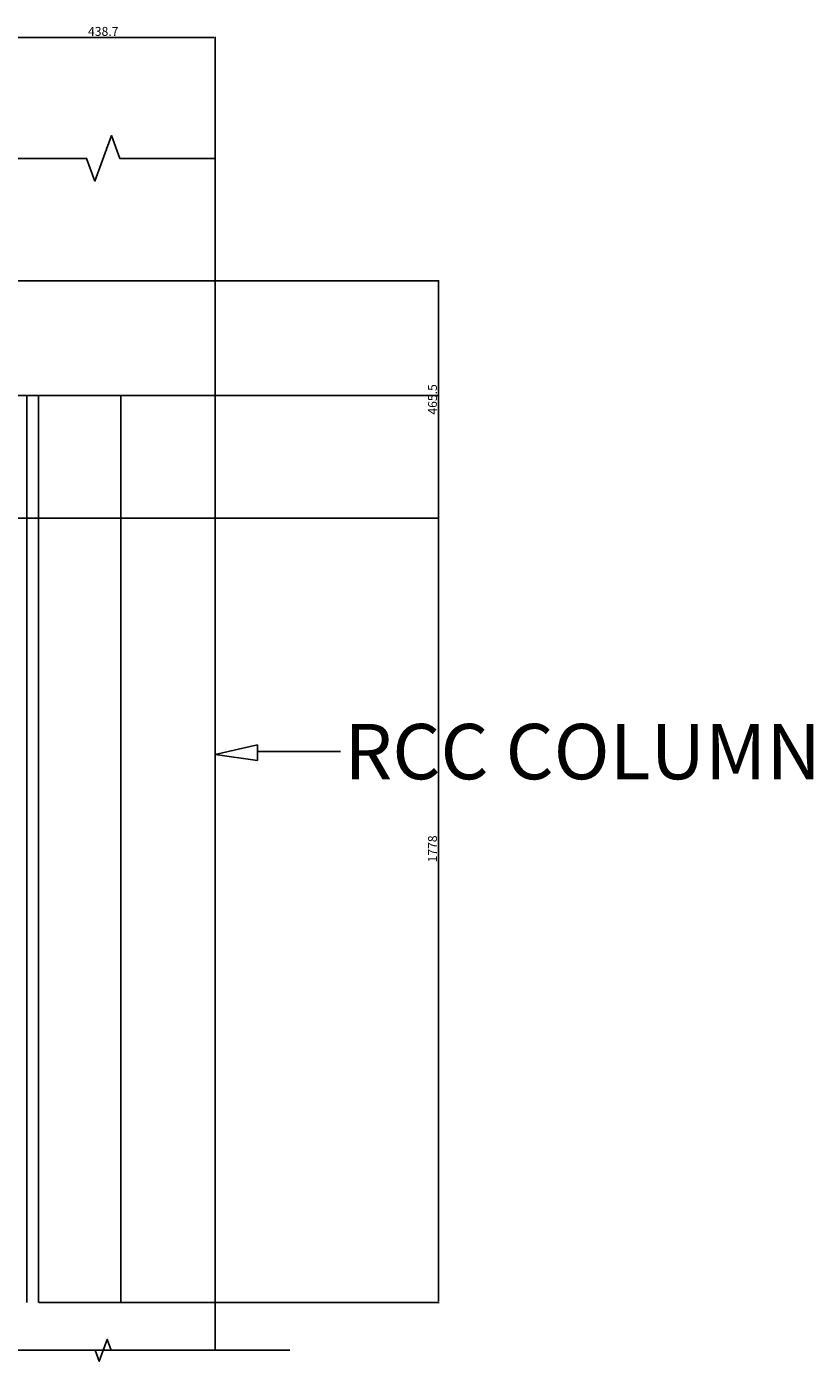
# Model space of a CAD drawing. Units: millimetres. Extents: x 498 to 8860, y -426 to 8717.
# Tile 4 of 9: x 7317 to 8860, y 733 to 3349. Entities that reach past the tile are written whole.
import ezdxf

# ---------------------------------------------------------------- set-up
doc = ezdxf.new("R2010")
doc.units = ezdxf.units.MM
for name, color, linetype, lineweight in [('A-ANNO-DIMS', 2, 'Continuous', 18), ('A-ANNO-TEXT', 3, 'Continuous', 18), ('A-DETL', 7, 'Continuous', 25)]:
    doc.layers.add(name, color=color, linetype=linetype, lineweight=lineweight)
doc.styles.get("Standard").update_dxf_attribs({"font": 'arial.ttf'})
doc.dimstyles.new('ISO-25', dxfattribs={"dimtxt": 17.5, "dimasz": 2.5, "dimexe": 1.25, "dimexo": 0.625, "dimtad": 1, "dimdec": 0, "dimtxsty": 'Standard', "dimcen": 2.5, "dimadec": 0, "dimazin": 0, "dimtfac": 1, "dimtdec": 0, "dimtmove": 0, "dimatfit": 3, "dimfxl": 1, "dimarcsym": 0})

# ---------------------------------------------------------------- blocks, each defined once
blk = doc.blocks.new('*D68')
at = {"layer": 'A-ANNO-DIMS', "color": 0, "lineweight": -2, "transparency": 16777216}
for p, q in [((7248.3, 2851.2), (8125.9, 2851.2)), ((8124.6, 2388.2), (8124.6, 2848.7)), ((5760.1, 2385.7), (8125.9, 2385.7))]:
    blk.add_line(p, q, dxfattribs=at)
at = {"layer": 'A-ANNO-DIMS', "color": 0, "transparency": 16777216}
for points in [[(8124.2, 2848.7), (8125, 2848.7), (8124.6, 2851.2)], [(8124.2, 2388.2), (8125, 2388.2), (8124.6, 2385.7)]]:
    blk.add_solid(points, dxfattribs=at)
at = {"layer": 'Defpoints', "color": 0, "transparency": 16777216}
for p in [(7247.7, 2851.2), (8124.6, 2851.2), (5759.5, 2385.7)]:
    blk.add_point(p, dxfattribs=at)
at = {"layer": 'A-ANNO-DIMS', "color": 0, "transparency": 16777216, "insert": (8115.1, 2618.5), "char_height": 17.5, "attachment_point": 5, "rotation": 90}
blk.add_mtext('465.5', dxfattribs=at)
blk = doc.blocks.new('*D69')
at = {"layer": 'A-ANNO-DIMS', "color": 0, "lineweight": -2, "transparency": 16777216}
for p, q in [((7247.7, 3091.6), (7247.7, 3329.3)), ((7250.2, 3328.1), (7683.9, 3328.1)), ((7686.4, 3091.6), (7686.4, 3329.3))]:
    blk.add_line(p, q, dxfattribs=at)
at = {"layer": 'A-ANNO-DIMS', "color": 0, "transparency": 16777216}
for points in [[(7250.2, 3328.5), (7250.2, 3327.6), (7247.7, 3328.1)], [(7683.9, 3328.5), (7683.9, 3327.6), (7686.4, 3328.1)]]:
    blk.add_solid(points, dxfattribs=at)
at = {"layer": 'Defpoints', "color": 0, "transparency": 16777216}
for p in [(7686.4, 3328.1), (7247.7, 3090.9), (7686.4, 3090.9)]:
    blk.add_point(p, dxfattribs=at)
at = {"layer": 'A-ANNO-DIMS', "color": 0, "transparency": 16777216, "insert": (7467.1, 3337.6), "char_height": 17.5, "attachment_point": 5}
blk.add_mtext('438.7', dxfattribs=at)
blk = doc.blocks.new('*D71')
at = {"layer": 'A-ANNO-DIMS', "color": 0, "lineweight": -2, "transparency": 16777216}
for p, q in [((7340.7, 2626.5), (8125.9, 2626.5)), ((8124.6, 2624), (8124.6, 850.9)), ((7340.7, 848.4), (8125.9, 848.4))]:
    blk.add_line(p, q, dxfattribs=at)
at = {"layer": 'A-ANNO-DIMS', "color": 0, "transparency": 16777216}
for points in [[(8124.2, 2624), (8125, 2624), (8124.6, 2626.5)], [(8124.2, 850.9), (8125, 850.9), (8124.6, 848.4)]]:
    blk.add_solid(points, dxfattribs=at)
at = {"layer": 'Defpoints', "color": 0, "transparency": 16777216}
for p in [(7340.1, 2626.5), (7340.1, 848.4), (8124.6, 848.4)]:
    blk.add_point(p, dxfattribs=at)
at = {"layer": 'A-ANNO-DIMS', "color": 0, "transparency": 16777216, "insert": (8115.1, 1737.4), "char_height": 17.5, "attachment_point": 5, "rotation": 90}
blk.add_mtext('1778', dxfattribs=at)

msp = doc.modelspace()

# ---------------------------------------------------------------- linework, layer by layer
at = {"layer": 'A-DETL'}
for p, q in [((7686.422, 754.555), (7686.422, 3090.936)), ((7247.72, 2626.504), (7686.422, 2626.504)), ((7316.989, 848.389), (7316.989, 2626.504)), ((7340.079, 848.389), (7340.079, 2626.504)), ((7501.706, 848.389), (7501.706, 2626.504)), ((7686.422, 1922.746), (7769.482, 1941.282)), ((7769.482, 1928.453), (7769.482, 1941.282)), ((7769.482, 1941.282), (7769.482, 1910.44)), ((7769.482, 1910.44), (7686.422, 1922.746)), ((7932.127, 1928.453), (7769.482, 1928.453)), ((7247.72, 754.555), (7686.422, 754.555))]:
    msp.add_line(p, q, dxfattribs=at)
for points in [[(7247.72, 3090.936), (7434.589, 3090.936), (7450.83, 3046.314), (7483.312, 3135.559), (7499.554, 3090.936), (7686.422, 3090.936)], [(7095.919, 754.555), (7451.409, 754.555), (7459.24, 733.039), (7474.902, 776.07), (7482.733, 754.555), (7833.194, 754.555)]]:
    msp.add_lwpolyline(points, dxfattribs=at)

# ---------------------------------------------------------------- texts
at = {"layer": 'A-ANNO-TEXT'}
msp.add_text('RCC COLUMN', height=108.4825, dxfattribs=at).set_placement((7940.013, 1873.944))

# ---------------------------------------------------------------- dimensions: what is measured, and where the dimension line sits
at = {"layer": 'A-ANNO-DIMS'}
dim = msp.add_linear_dim(base=(7686.422, 3328.059), p1=(7247.72, 3090.936), p2=(7686.422, 3090.936), dimstyle='ISO-25', override={"dimdec": 1, "dimlfac": 1, "dimrnd": 0, "dimzin": 0, "dimdsep": 46, "dimlunit": 2}, dxfattribs=at)
dim.commit()
dim.dimension.update_dxf_attribs({"geometry": '*D69', "text_midpoint": (7467.071, 3337.625)})
for base, p1, p2, override, picture, middle in [((8124.627, 2851.24), (5759.508, 2385.702), (7247.72, 2851.24), {"dimdec": 1, "dimlfac": 1, "dimrnd": 0, "dimzin": 0, "dimdsep": 46, "dimlunit": 2}, '*D68', (8115.067, 2618.471)), ((8124.627, 848.389), (7340.079, 2626.504), (7340.079, 848.389), {"dimdec": 0, "dimlfac": 1, "dimrnd": 0, "dimzin": 0, "dimdsep": 46, "dimlunit": 2}, '*D71', (8115.067, 1737.446))]:
    dim = msp.add_linear_dim(base=base, p1=p1, p2=p2, angle=90, dimstyle='ISO-25', override=override, dxfattribs=at)
    dim.commit()
    dim.dimension.update_dxf_attribs({"geometry": picture, "text_midpoint": middle})

doc.saveas('drawing.dxf')
